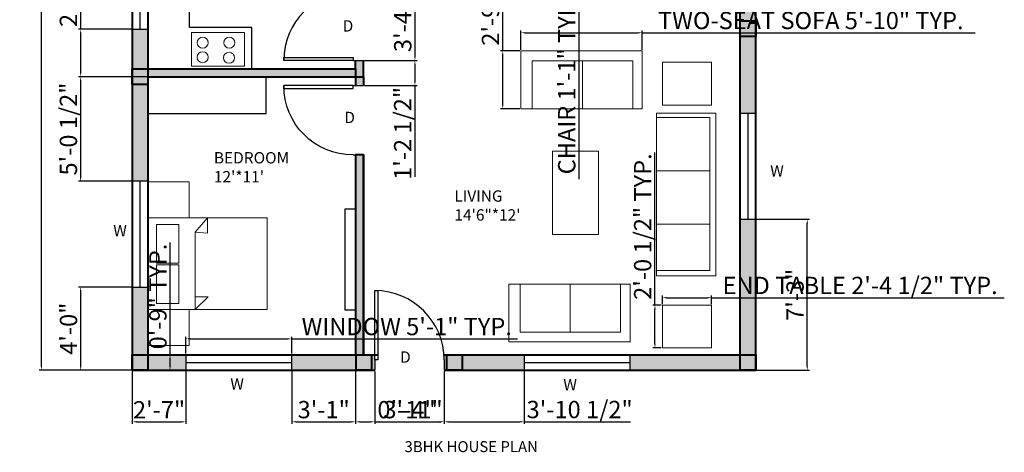
# Model space of a CAD drawing. Units: inches. Extents: x 1628 to 2197, y 2073 to 2736.
# Tile 1 of 3: x 1628 to 2197, y 2073 to 2323. Entities that reach past the tile are written whole.
import ezdxf

# ---------------------------------------------------------------- set-up
doc = ezdxf.new("R2010")
doc.units = ezdxf.units.IN
for name, color, linetype, lineweight in [('A-ANNO-DIMS', 2, 'Continuous', 18), ('A-ANNO-IDEN', 7, 'Continuous', 18), ('A-ANNO-TEXT', 7, 'Continuous', 25), ('A-AREA-IDEN', 7, 'Continuous', 18), ('A-COLS', 7, 'Continuous', 40), ('A-COLS-PATT', 8, 'Continuous', 13), ('A-EQPM', 8, 'Continuous', 18), ('A-FLOR-CASE', 8, 'Continuous', 25), ('A-FURN', 8, 'Continuous', 18), ('A-WALL-PATT', 152, 'Continuous', 13), ('bed', 210, 'Continuous', 18), ('door', 52, 'Continuous', 25), ('sofa', 190, 'Continuous', 18), ('wall', 151, 'Continuous', 40), ('window', 20, 'Continuous', 25)]:
    doc.layers.add(name, color=color, linetype=linetype, lineweight=lineweight)
doc.styles.get("Standard").update_dxf_attribs({"font": 'arial.ttf'})
doc.dimstyles.new('ISO-25', dxfattribs={"dimtxt": 10, "dimasz": 2.5, "dimexe": 1.25, "dimexo": 0.625, "dimtad": 1, "dimdec": 0, "dimlunit": 4, "dimtxsty": 'Standard', "dimcen": 2.5, "dimadec": 0, "dimazin": 0, "dimtfac": 1, "dimtdec": 0, "dimtmove": 0, "dimatfit": 3, "dimfxl": 1, "dimarcsym": 0})

# ---------------------------------------------------------------- blocks, each defined once
blk = doc.blocks.new('*U2')
for p, q in [((0, 0), (0, -6)), ((40, 0), (40, -6))]:
    blk.add_line(p, q)
blk.add_lwpolyline([(0, 0), (0, 40), (1.75, 40), (1.75, 0)], close=True)
blk.add_arc((0, 0), 40, 0, 90)
blk = doc.blocks.new('*D6')
at = {"layer": 'A-ANNO-DIMS', "color": 0, "lineweight": -2, "transparency": 16777216}
for p, q in [((1692.49, 2600.7), (1639.45, 2600.7)), ((1640.7, 2123.2), (1640.7, 2598.2)), ((1692.49, 2120.7), (1639.45, 2120.7))]:
    blk.add_line(p, q, dxfattribs=at)
at = {"layer": 'A-ANNO-DIMS', "color": 0, "transparency": 16777216}
for points in [[(1640.28, 2598.2), (1641.11, 2598.2), (1640.7, 2600.7)], [(1640.28, 2123.2), (1641.11, 2123.2), (1640.7, 2120.7)]]:
    blk.add_solid(points, dxfattribs=at)
at = {"layer": 'Defpoints', "color": 0, "transparency": 16777216}
for p in [(1640.7, 2600.7), (1693.11, 2600.7), (1693.11, 2120.7)]:
    blk.add_point(p, dxfattribs=at)
at = {"layer": 'A-ANNO-DIMS', "color": 0, "transparency": 16777216, "insert": (1634.96, 2360.7), "char_height": 10, "attachment_point": 5, "rotation": 90}
blk.add_mtext("40'", dxfattribs=at)
blk = doc.blocks.new('BED-DOUBLE-WITH-NIGHTSTANDS')
for p, q in [((27.37, 65.6), (34.42, 73.72)), ((34.42, 73.72), (34.42, 64.86)), ((27.37, 28.24), (27.37, 65.6)), ((34.42, 64.86), (27.37, 65.6)), ((27.37, 28.24), (27.37, 20.94)), ((27.37, 20.94), (34.96, 28.24)), ((34.96, 28.24), (27.37, 28.24))]:
    blk.add_line(p, q)
for points in [[(0, 73.72), (23.98, 73.72), (23.98, 94.66), (0, 94.66)], [(0, 20.94), (68.84, 20.94), (68.84, 73.72), (0, 73.72)], [(4.97, 47.66), (17.93, 47.66), (17.93, 70.03), (4.97, 70.03)], [(4.97, 24.36), (17.93, 24.36), (17.93, 46.73), (4.97, 46.73)], [(0, 0), (23.98, 0), (23.98, 20.94), (0, 20.94)]]:
    blk.add_lwpolyline(points, close=True)
blk = doc.blocks.new('SOFA-TWO-SEAT')
for p, q in [((0, 0), (0, 33.36)), ((0, 33.36), (70, 33.36)), ((70, 33.36), (70, 0)), ((35.49, 27.75), (35.49, 0)), ((6.45, 0), (0, 0)), ((70, 0), (54.71, 0))]:
    blk.add_line(p, q)
blk.add_lwpolyline([(64.53, 27.75), (6.45, 27.75), (6.45, 0), (64.53, 0)], close=True)
blk = doc.blocks.new('TABLE-END')
blk.add_lwpolyline([(28.46, 0), (0, 0), (0, 24.71), (28.46, 24.71)], close=True)
blk = doc.blocks.new('WINDOW-61IN')
blk.add_line((0, 4.5), (61.1, 4.5))
blk.add_lwpolyline([(0, 0), (61.1, 0), (61.1, 9), (0, 9)], close=True)
blk = doc.blocks.new('COLUMN-9X9')
blk.add_lwpolyline([(0, 9), (9, 9), (9, 0), (0, 0)], close=True)
blk = doc.blocks.new('*D15')
at = {"layer": 'A-ANNO-DIMS', "color": 0, "lineweight": -2, "transparency": 16777216}
for p, q in [((1724.14, 2130.33), (1724.14, 2140.12)), ((1726.64, 2138.87), (1782.75, 2138.87)), ((1785.25, 2130.33), (1785.25, 2140.12)), ((1785.25, 2138.87), (1915.54, 2138.87))]:
    blk.add_line(p, q, dxfattribs=at)
at = {"layer": 'A-ANNO-DIMS', "color": 0, "transparency": 16777216}
for points in [[(1726.64, 2139.28), (1726.64, 2138.45), (1724.14, 2138.87)], [(1782.75, 2139.28), (1782.75, 2138.45), (1785.25, 2138.87)]]:
    blk.add_solid(points, dxfattribs=at)
at = {"layer": 'Defpoints', "color": 0, "transparency": 16777216}
for p in [(1785.25, 2138.87), (1724.14, 2129.7), (1785.25, 2129.7)]:
    blk.add_point(p, dxfattribs=at)
at = {"layer": 'A-ANNO-DIMS', "color": 0, "transparency": 16777216, "insert": (1851.64, 2144.67), "char_height": 10, "attachment_point": 5}
blk.add_mtext('WINDOW 5\'-1" TYP.', dxfattribs=at)
blk = doc.blocks.new('*D16')
at = {"layer": 'A-ANNO-DIMS', "color": 0, "lineweight": -2, "transparency": 16777216}
for p, q in [((1714.98, 2129.7), (1714.98, 2194.41)), ((1723.52, 2129.7), (1713.73, 2129.7)), ((1714.98, 2123.2), (1714.98, 2127.2)), ((1723.52, 2120.7), (1713.73, 2120.7))]:
    blk.add_line(p, q, dxfattribs=at)
at = {"layer": 'A-ANNO-DIMS', "color": 0, "transparency": 16777216}
for points in [[(1714.56, 2127.2), (1715.39, 2127.2), (1714.98, 2129.7)], [(1714.56, 2123.2), (1715.39, 2123.2), (1714.98, 2120.7)]]:
    blk.add_solid(points, dxfattribs=at)
at = {"layer": 'Defpoints', "color": 0, "transparency": 16777216}
for p in [(1714.98, 2129.7), (1724.14, 2129.7), (1724.14, 2120.7)]:
    blk.add_point(p, dxfattribs=at)
at = {"layer": 'A-ANNO-DIMS', "color": 0, "transparency": 16777216, "insert": (1709.25, 2163.3), "char_height": 10, "attachment_point": 5, "rotation": 90}
blk.add_mtext('0\'-9" TYP.', dxfattribs=at)
blk = doc.blocks.new('*D17')
at = {"layer": 'A-ANNO-DIMS', "color": 0, "lineweight": -2, "transparency": 16777216}
for p, q in [((1949.73, 2356.08), (1952.33, 2356.08)), ((1951.08, 2353.58), (1951.08, 2345.41)), ((1949.73, 2342.91), (1952.33, 2342.91)), ((1951.08, 2342.91), (1951.08, 2230.98))]:
    blk.add_line(p, q, dxfattribs=at)
at = {"layer": 'A-ANNO-DIMS', "color": 0, "transparency": 16777216}
for points in [[(1950.66, 2353.58), (1951.5, 2353.58), (1951.08, 2356.08)], [(1950.66, 2345.41), (1951.5, 2345.41), (1951.08, 2342.91)]]:
    blk.add_solid(points, dxfattribs=at)
at = {"layer": 'Defpoints', "color": 0, "transparency": 16777216}
for p in [(1949.11, 2356.08), (1949.11, 2342.91), (1951.08, 2342.91)]:
    blk.add_point(p, dxfattribs=at)
at = {"layer": 'A-ANNO-DIMS', "color": 0, "transparency": 16777216, "insert": (1945.29, 2285.7), "char_height": 10, "attachment_point": 5, "rotation": 90}
blk.add_mtext('CHAIR 1\'-1" TYP.', dxfattribs=at)
blk = doc.blocks.new('*D21')
at = {"layer": 'A-ANNO-DIMS', "color": 0, "lineweight": -2, "transparency": 16777216}
for p, q in [((1999.21, 2158.97), (1999.21, 2163.86)), ((2001.71, 2162.61), (2025.17, 2162.61)), ((2027.67, 2158.97), (2027.67, 2163.86)), ((2027.67, 2162.61), (2196.66, 2162.61))]:
    blk.add_line(p, q, dxfattribs=at)
at = {"layer": 'A-ANNO-DIMS', "color": 0, "transparency": 16777216}
for points in [[(2001.71, 2163.03), (2001.71, 2162.2), (1999.21, 2162.61)], [(2025.17, 2163.03), (2025.17, 2162.2), (2027.67, 2162.61)]]:
    blk.add_solid(points, dxfattribs=at)
at = {"layer": 'Defpoints', "color": 0, "transparency": 16777216}
for p in [(2027.67, 2162.61), (1999.21, 2158.35), (2027.67, 2158.35)]:
    blk.add_point(p, dxfattribs=at)
at = {"layer": 'A-ANNO-DIMS', "color": 0, "transparency": 16777216, "insert": (2113.41, 2168.41), "char_height": 10, "attachment_point": 5}
blk.add_mtext('END TABLE 2\'-4 1/2" TYP.', dxfattribs=at)
blk = doc.blocks.new('*D22')
at = {"layer": 'A-ANNO-DIMS', "color": 0, "lineweight": -2, "transparency": 16777216}
for p, q in [((1994.94, 2158.35), (1994.94, 2246.52)), ((1998.58, 2158.35), (1993.69, 2158.35)), ((1994.94, 2136.14), (1994.94, 2155.85)), ((1998.58, 2133.64), (1993.69, 2133.64))]:
    blk.add_line(p, q, dxfattribs=at)
at = {"layer": 'A-ANNO-DIMS', "color": 0, "transparency": 16777216}
for points in [[(1994.52, 2155.85), (1995.36, 2155.85), (1994.94, 2158.35)], [(1994.52, 2136.14), (1995.36, 2136.14), (1994.94, 2133.64)]]:
    blk.add_solid(points, dxfattribs=at)
at = {"layer": 'Defpoints', "color": 0, "transparency": 16777216}
for p in [(1994.94, 2158.35), (1999.21, 2158.35), (1999.21, 2133.64)]:
    blk.add_point(p, dxfattribs=at)
at = {"layer": 'A-ANNO-DIMS', "color": 0, "transparency": 16777216, "insert": (1989.14, 2203.68), "char_height": 10, "attachment_point": 5, "rotation": 90}
blk.add_mtext('2\'-0 1/2" TYP.', dxfattribs=at)
blk = doc.blocks.new('*D23')
at = {"layer": 'A-ANNO-DIMS', "color": 0, "lineweight": -2, "transparency": 16777216}
for p, q in [((1917.57, 2305.72), (1917.57, 2316.85)), ((1920.07, 2315.6), (1985.07, 2315.6)), ((1987.57, 2305.72), (1987.57, 2316.85)), ((1987.57, 2315.6), (2179.82, 2315.6))]:
    blk.add_line(p, q, dxfattribs=at)
at = {"layer": 'A-ANNO-DIMS', "color": 0, "transparency": 16777216}
for points in [[(1920.07, 2316.01), (1920.07, 2315.18), (1917.57, 2315.6)], [(1985.07, 2316.01), (1985.07, 2315.18), (1987.57, 2315.6)]]:
    blk.add_solid(points, dxfattribs=at)
at = {"layer": 'Defpoints', "color": 0, "transparency": 16777216}
for p in [(1987.57, 2315.6), (1917.57, 2305.1), (1987.57, 2305.1)]:
    blk.add_point(p, dxfattribs=at)
at = {"layer": 'A-ANNO-DIMS', "color": 0, "transparency": 16777216, "insert": (2084.94, 2321.4), "char_height": 10, "attachment_point": 5}
blk.add_mtext('TWO-SEAT SOFA 5\'-10" TYP.', dxfattribs=at)
blk = doc.blocks.new('*D24')
at = {"layer": 'A-ANNO-DIMS', "color": 0, "lineweight": -2, "transparency": 16777216}
for p, q in [((1907.07, 2305.1), (1907.07, 2393.27)), ((1916.95, 2305.1), (1905.82, 2305.1)), ((1907.07, 2274.24), (1907.07, 2302.6)), ((1916.95, 2271.74), (1905.82, 2271.74))]:
    blk.add_line(p, q, dxfattribs=at)
at = {"layer": 'A-ANNO-DIMS', "color": 0, "transparency": 16777216}
for points in [[(1906.65, 2302.6), (1907.49, 2302.6), (1907.07, 2305.1)], [(1906.65, 2274.24), (1907.49, 2274.24), (1907.07, 2271.74)]]:
    blk.add_solid(points, dxfattribs=at)
at = {"layer": 'Defpoints', "color": 0, "transparency": 16777216}
for p in [(1907.07, 2305.1), (1917.57, 2305.1), (1917.57, 2271.74)]:
    blk.add_point(p, dxfattribs=at)
at = {"layer": 'A-ANNO-DIMS', "color": 0, "transparency": 16777216, "insert": (1901.28, 2350.44), "char_height": 10, "attachment_point": 5, "rotation": 90}
blk.add_mtext('2\'-9 1/2" TYP.', dxfattribs=at)
blk = doc.blocks.new('*D28')
at = {"layer": 'A-ANNO-DIMS', "color": 0, "lineweight": -2, "transparency": 16777216}
for p, q in [((1693.11, 2120.08), (1693.11, 2089.7)), ((1724.14, 2120.08), (1724.14, 2089.7)), ((1695.61, 2090.95), (1721.64, 2090.95))]:
    blk.add_line(p, q, dxfattribs=at)
at = {"layer": 'A-ANNO-DIMS', "color": 0, "transparency": 16777216}
for points in [[(1695.61, 2091.37), (1695.61, 2090.54), (1693.11, 2090.95)], [(1721.64, 2091.37), (1721.64, 2090.54), (1724.14, 2090.95)]]:
    blk.add_solid(points, dxfattribs=at)
at = {"layer": 'Defpoints', "color": 0, "transparency": 16777216}
for p in [(1693.11, 2120.7), (1724.14, 2120.7), (1724.14, 2090.95)]:
    blk.add_point(p, dxfattribs=at)
at = {"layer": 'A-ANNO-DIMS', "color": 0, "transparency": 16777216, "insert": (1708.63, 2096.6), "char_height": 10, "attachment_point": 5}
blk.add_mtext('2\'-7"', dxfattribs=at)
blk = doc.blocks.new('*D29')
at = {"layer": 'A-ANNO-DIMS', "color": 0, "lineweight": -2, "transparency": 16777216}
for p, q in [((1822.11, 2129.08), (1822.11, 2089.7)), ((1785.25, 2120.08), (1785.25, 2089.7)), ((1787.75, 2090.95), (1819.61, 2090.95))]:
    blk.add_line(p, q, dxfattribs=at)
at = {"layer": 'A-ANNO-DIMS', "color": 0, "transparency": 16777216}
for points in [[(1787.75, 2091.37), (1787.75, 2090.54), (1785.25, 2090.95)], [(1819.61, 2091.37), (1819.61, 2090.54), (1822.11, 2090.95)]]:
    blk.add_solid(points, dxfattribs=at)
at = {"layer": 'Defpoints', "color": 0, "transparency": 16777216}
for p in [(1822.11, 2129.7), (1785.25, 2120.7), (1822.11, 2090.95)]:
    blk.add_point(p, dxfattribs=at)
at = {"layer": 'A-ANNO-DIMS', "color": 0, "transparency": 16777216, "insert": (1803.68, 2096.69), "char_height": 10, "attachment_point": 5}
blk.add_mtext('3\'-1"', dxfattribs=at)
blk = doc.blocks.new('*D30')
at = {"layer": 'A-ANNO-DIMS', "color": 0, "lineweight": -2, "transparency": 16777216}
for p, q in [((1822.11, 2129.08), (1822.11, 2089.7)), ((1833.23, 2120.08), (1833.23, 2089.7)), ((1824.61, 2090.95), (1830.73, 2090.95)), ((1833.23, 2090.95), (1871.33, 2090.95))]:
    blk.add_line(p, q, dxfattribs=at)
at = {"layer": 'A-ANNO-DIMS', "color": 0, "transparency": 16777216}
for points in [[(1824.61, 2091.37), (1824.61, 2090.54), (1822.11, 2090.95)], [(1830.73, 2091.37), (1830.73, 2090.54), (1833.23, 2090.95)]]:
    blk.add_solid(points, dxfattribs=at)
at = {"layer": 'Defpoints', "color": 0, "transparency": 16777216}
for p in [(1822.11, 2129.7), (1833.23, 2120.7), (1833.23, 2090.95)]:
    blk.add_point(p, dxfattribs=at)
at = {"layer": 'A-ANNO-DIMS', "color": 0, "transparency": 16777216, "insert": (1853.53, 2096.68), "char_height": 10, "attachment_point": 5}
blk.add_mtext('0\'-11"', dxfattribs=at)
blk = doc.blocks.new('*D31')
at = {"layer": 'A-ANNO-DIMS', "color": 0, "lineweight": -2, "transparency": 16777216}
for p, q in [((1833.23, 2120.08), (1833.23, 2089.7)), ((1873.23, 2120.08), (1873.23, 2089.7)), ((1835.73, 2090.95), (1870.73, 2090.95))]:
    blk.add_line(p, q, dxfattribs=at)
at = {"layer": 'A-ANNO-DIMS', "color": 0, "transparency": 16777216}
for points in [[(1835.73, 2091.37), (1835.73, 2090.54), (1833.23, 2090.95)], [(1870.73, 2091.37), (1870.73, 2090.54), (1873.23, 2090.95)]]:
    blk.add_solid(points, dxfattribs=at)
at = {"layer": 'Defpoints', "color": 0, "transparency": 16777216}
for p in [(1833.23, 2120.7), (1873.23, 2120.7), (1873.23, 2090.95)]:
    blk.add_point(p, dxfattribs=at)
at = {"layer": 'A-ANNO-DIMS', "color": 0, "transparency": 16777216, "insert": (1853.23, 2096.69), "char_height": 10, "attachment_point": 5}
blk.add_mtext('3\'-4"', dxfattribs=at)
blk = doc.blocks.new('*D32')
at = {"layer": 'A-ANNO-DIMS', "color": 0, "lineweight": -2, "transparency": 16777216}
for p, q in [((1873.23, 2120.08), (1873.23, 2089.7)), ((1919.51, 2120.08), (1919.51, 2089.7)), ((1875.73, 2090.95), (1917.01, 2090.95)), ((1919.51, 2090.95), (1980.91, 2090.95))]:
    blk.add_line(p, q, dxfattribs=at)
at = {"layer": 'A-ANNO-DIMS', "color": 0, "transparency": 16777216}
for points in [[(1875.73, 2091.37), (1875.73, 2090.54), (1873.23, 2090.95)], [(1917.01, 2091.37), (1917.01, 2090.54), (1919.51, 2090.95)]]:
    blk.add_solid(points, dxfattribs=at)
at = {"layer": 'Defpoints', "color": 0, "transparency": 16777216}
for p in [(1873.23, 2120.7), (1919.51, 2120.7), (1919.51, 2090.95)]:
    blk.add_point(p, dxfattribs=at)
at = {"layer": 'A-ANNO-DIMS', "color": 0, "transparency": 16777216, "insert": (1951.46, 2096.75), "char_height": 10, "attachment_point": 5}
blk.add_mtext('3\'-10 1/2"', dxfattribs=at)
blk = doc.blocks.new('*D33')
at = {"layer": 'A-ANNO-DIMS', "color": 0, "lineweight": -2, "transparency": 16777216}
for p, q in [((1692.49, 2168.74), (1662.11, 2168.74)), ((1663.36, 2123.2), (1663.36, 2166.24)), ((1692.49, 2120.7), (1662.11, 2120.7))]:
    blk.add_line(p, q, dxfattribs=at)
at = {"layer": 'A-ANNO-DIMS', "color": 0, "transparency": 16777216}
for points in [[(1662.94, 2166.24), (1663.78, 2166.24), (1663.36, 2168.74)], [(1662.94, 2123.2), (1663.78, 2123.2), (1663.36, 2120.7)]]:
    blk.add_solid(points, dxfattribs=at)
at = {"layer": 'Defpoints', "color": 0, "transparency": 16777216}
for p in [(1663.36, 2168.74), (1693.11, 2168.74), (1693.11, 2120.7)]:
    blk.add_point(p, dxfattribs=at)
at = {"layer": 'A-ANNO-DIMS', "color": 0, "transparency": 16777216, "insert": (1657.63, 2144.72), "char_height": 10, "attachment_point": 5, "rotation": 90}
blk.add_mtext('4\'-0"', dxfattribs=at)
blk = doc.blocks.new('*D34')
at = {"layer": 'A-ANNO-DIMS', "color": 0, "lineweight": -2, "transparency": 16777216}
for p, q in [((1701.49, 2290.2), (1662.11, 2290.2)), ((1663.36, 2232.34), (1663.36, 2287.7)), ((1692.49, 2229.84), (1662.11, 2229.84))]:
    blk.add_line(p, q, dxfattribs=at)
at = {"layer": 'A-ANNO-DIMS', "color": 0, "transparency": 16777216}
for points in [[(1662.94, 2287.7), (1663.78, 2287.7), (1663.36, 2290.2)], [(1662.94, 2232.34), (1663.78, 2232.34), (1663.36, 2229.84)]]:
    blk.add_solid(points, dxfattribs=at)
at = {"layer": 'Defpoints', "color": 0, "transparency": 16777216}
for p in [(1663.36, 2290.2), (1702.11, 2290.2), (1693.11, 2229.84)]:
    blk.add_point(p, dxfattribs=at)
at = {"layer": 'A-ANNO-DIMS', "color": 0, "transparency": 16777216, "insert": (1657.57, 2260.02), "char_height": 10, "attachment_point": 5, "rotation": 90}
blk.add_mtext('5\'-0 1/2"', dxfattribs=at)
blk = doc.blocks.new('*D35')
at = {"layer": 'A-ANNO-DIMS', "color": 0, "lineweight": -2, "transparency": 16777216}
for p, q in [((1663.36, 2317.65), (1663.36, 2371.45)), ((1692.49, 2317.65), (1662.11, 2317.65)), ((1663.36, 2292.7), (1663.36, 2315.15)), ((1701.49, 2290.2), (1662.11, 2290.2))]:
    blk.add_line(p, q, dxfattribs=at)
at = {"layer": 'A-ANNO-DIMS', "color": 0, "transparency": 16777216}
for points in [[(1662.94, 2315.15), (1663.78, 2315.15), (1663.36, 2317.65)], [(1662.94, 2292.7), (1663.78, 2292.7), (1663.36, 2290.2)]]:
    blk.add_solid(points, dxfattribs=at)
at = {"layer": 'Defpoints', "color": 0, "transparency": 16777216}
for p in [(1663.36, 2317.65), (1693.11, 2317.65), (1702.11, 2290.2)]:
    blk.add_point(p, dxfattribs=at)
at = {"layer": 'A-ANNO-DIMS', "color": 0, "transparency": 16777216, "insert": (1657.56, 2345.8), "char_height": 10, "attachment_point": 5, "rotation": 90}
blk.add_mtext('2\'-3 1/2"', dxfattribs=at)
blk = doc.blocks.new('*D41')
at = {"layer": 'A-ANNO-DIMS', "color": 0, "lineweight": -2, "transparency": 16777216}
for p, q in [((2053.74, 2207.91), (2084.11, 2207.91)), ((2082.86, 2123.2), (2082.86, 2205.41)), ((2053.74, 2120.7), (2084.11, 2120.7))]:
    blk.add_line(p, q, dxfattribs=at)
at = {"layer": 'A-ANNO-DIMS', "color": 0, "transparency": 16777216}
for points in [[(2082.44, 2205.41), (2083.28, 2205.41), (2082.86, 2207.91)], [(2082.44, 2123.2), (2083.28, 2123.2), (2082.86, 2120.7)]]:
    blk.add_solid(points, dxfattribs=at)
at = {"layer": 'Defpoints', "color": 0, "transparency": 16777216}
for p in [(2053.11, 2207.91), (2082.86, 2207.91), (2053.11, 2120.7)]:
    blk.add_point(p, dxfattribs=at)
at = {"layer": 'A-ANNO-DIMS', "color": 0, "transparency": 16777216, "insert": (2077.13, 2164.31), "char_height": 10, "attachment_point": 5, "rotation": 90}
blk.add_mtext('7\'-3"', dxfattribs=at)
blk = doc.blocks.new('*D52')
at = {"layer": 'A-ANNO-DIMS', "color": 0, "lineweight": -2, "transparency": 16777216}
for p, q in [((1827.24, 2299.52), (1857.61, 2299.52)), ((1856.36, 2297.02), (1856.36, 2287.58)), ((1827.24, 2285.08), (1857.61, 2285.08)), ((1856.36, 2285.08), (1856.36, 2232.39))]:
    blk.add_line(p, q, dxfattribs=at)
at = {"layer": 'A-ANNO-DIMS', "color": 0, "transparency": 16777216}
for points in [[(1855.94, 2297.02), (1856.78, 2297.02), (1856.36, 2299.52)], [(1855.94, 2287.58), (1856.78, 2287.58), (1856.36, 2285.08)]]:
    blk.add_solid(points, dxfattribs=at)
at = {"layer": 'Defpoints', "color": 0, "transparency": 16777216}
for p in [(1826.61, 2299.52), (1826.61, 2285.08), (1856.36, 2285.08)]:
    blk.add_point(p, dxfattribs=at)
at = {"layer": 'A-ANNO-DIMS', "color": 0, "transparency": 16777216, "insert": (1850.57, 2257.49), "char_height": 10, "attachment_point": 5, "rotation": 90}
blk.add_mtext('1\'-2 1/2"', dxfattribs=at)
blk = doc.blocks.new('*D53')
at = {"layer": 'A-ANNO-DIMS', "color": 0, "lineweight": -2, "transparency": 16777216}
for p, q in [((1827.24, 2339.52), (1857.61, 2339.52)), ((1856.36, 2337.02), (1856.36, 2302.02)), ((1827.24, 2299.52), (1857.61, 2299.52))]:
    blk.add_line(p, q, dxfattribs=at)
at = {"layer": 'A-ANNO-DIMS', "color": 0, "transparency": 16777216}
for points in [[(1855.94, 2337.02), (1856.78, 2337.02), (1856.36, 2339.52)], [(1855.94, 2302.02), (1856.78, 2302.02), (1856.36, 2299.52)]]:
    blk.add_solid(points, dxfattribs=at)
at = {"layer": 'Defpoints', "color": 0, "transparency": 16777216}
for p in [(1826.61, 2339.52), (1826.61, 2299.52), (1856.36, 2299.52)]:
    blk.add_point(p, dxfattribs=at)
at = {"layer": 'A-ANNO-DIMS', "color": 0, "transparency": 16777216, "insert": (1850.63, 2319.52), "char_height": 10, "attachment_point": 5, "rotation": 90}
blk.add_mtext('3\'-4"', dxfattribs=at)

msp = doc.modelspace()

# ---------------------------------------------------------------- hatches: boundary and pattern name
at = {"layer": 'A-COLS-PATT'}
h = msp.add_hatch(color=256, dxfattribs=at)
h.dxf.hatch_style = 1
h.paths.add_polyline_path([(1702.11, 2600.7), (1693.11, 2600.7), (1693.11, 2591.7), (1702.11, 2591.7)])
h.paths.add_polyline_path([(1879.79, 2600.7), (1870.79, 2600.7), (1870.79, 2591.7), (1879.79, 2591.7)])
h.paths.add_polyline_path([(2053.11, 2600.7), (2044.11, 2600.7), (2044.11, 2591.7), (2053.11, 2591.7)])
h.paths.add_polyline_path([(1702.11, 2395.2), (1693.11, 2395.2), (1693.11, 2386.2), (1702.11, 2386.2)])
h.paths.add_polyline_path([(1826.61, 2395.2), (1817.61, 2395.2), (1817.61, 2386.2), (1826.61, 2386.2)])
h.paths.add_polyline_path([(1702.11, 2459.7), (1693.11, 2459.7), (1693.11, 2450.7), (1702.11, 2450.7)])
h.paths.add_polyline_path([(2053.11, 2459.7), (2044.11, 2459.7), (2044.11, 2455.2), (2053.11, 2455.2)])
h.paths.add_polyline_path([(2053.11, 2455.2), (2044.11, 2455.2), (2044.11, 2451.94), (2053.11, 2451.94)])
h.paths.add_polyline_path([(2053.11, 2460.94), (2044.11, 2460.94), (2044.11, 2459.7), (2053.11, 2459.7)])
h.paths.add_polyline_path([(2053.11, 2390.99), (2044.11, 2390.99), (2044.11, 2381.99), (2053.11, 2381.99)])
h.paths.add_polyline_path([(2053.11, 2322.52), (2044.11, 2322.52), (2044.11, 2313.52), (2053.11, 2313.52)])
h.paths.add_polyline_path([(1702.11, 2294.7), (1693.11, 2294.7), (1693.11, 2285.7), (1702.11, 2285.7)])
h.paths.add_polyline_path([(1702.11, 2129.7), (1693.11, 2129.7), (1693.11, 2120.7), (1702.11, 2120.7)])
h.paths.add_polyline_path([(1831.35, 2129.7), (1822.35, 2129.7), (1822.35, 2120.7), (1831.35, 2120.7)])
h.paths.add_polyline_path([(1883.72, 2129.7), (1874.72, 2129.7), (1874.72, 2120.7), (1883.72, 2120.7)])
h.paths.add_polyline_path([(2053.11, 2129.7), (2044.11, 2129.7), (2044.11, 2120.7), (2053.11, 2120.7)])
at = {"layer": 'A-WALL-PATT'}
h = msp.add_hatch(color=256, dxfattribs=at)
h.dxf.hatch_style = 1
h.paths.add_polyline_path([(1753.01, 2600.7), (1702.11, 2600.7), (1702.11, 2591.7), (1753.01, 2591.7)])
h.paths.add_polyline_path([(1870.79, 2600.7), (1814.12, 2600.7), (1814.12, 2591.7), (1870.79, 2591.7)])
h.paths.add_polyline_path([(1948.37, 2600.7), (1879.79, 2600.7), (1879.79, 2591.7), (1909.32, 2591.7), (1948.37, 2591.7)])
h.paths.add_polyline_path([(2044.11, 2600.7), (2009.47, 2600.7), (2009.47, 2591.7), (2044.11, 2591.7)])
h.paths.add_polyline_path([(2053.11, 2591.7), (2044.11, 2591.7), (2044.11, 2550.07), (2053.11, 2550.07)])
h.paths.add_polyline_path([(1702.11, 2591.7), (1693.11, 2591.7), (1693.11, 2549.95), (1702.11, 2549.95)])
h.paths.add_polyline_path([(1702.11, 2488.85), (1693.11, 2488.85), (1693.11, 2459.7), (1702.11, 2459.7)])
h.paths.add_polyline_path([(1828.05, 2459.7), (1702.11, 2459.7), (1702.11, 2455.2), (1733.61, 2455.2), (1792.11, 2455.2), (1828.05, 2455.2)])
h.paths.add_polyline_path([(1885.43, 2459.7), (1868.05, 2459.7), (1868.05, 2455.2), (1885.43, 2455.2)])
h.paths.add_polyline_path([(2053.11, 2488.97), (2044.11, 2488.97), (2044.11, 2474.68), (2044.11, 2460.94), (2053.11, 2460.94)])
h.paths.add_polyline_path([(2053.11, 2451.94), (2044.11, 2451.94), (2044.11, 2437.29), (2053.11, 2437.29)])
h.paths.add_polyline_path([(2053.11, 2414.88), (2044.11, 2414.88), (2044.11, 2390.99), (2053.11, 2390.99)])
h.paths.add_polyline_path([(2044.11, 2459.7), (1925.43, 2459.7), (1925.43, 2455.2), (2044.11, 2455.2)])
h.paths.add_polyline_path([(2053.11, 2381.99), (2044.11, 2381.99), (2044.11, 2322.52), (2053.11, 2322.52)])
h.paths.add_polyline_path([(1919.51, 2129.7), (1883.72, 2129.7), (1883.72, 2120.7), (1919.51, 2120.7)])
h.paths.add_polyline_path([(2044.11, 2129.7), (1980.61, 2129.7), (1980.61, 2120.7), (2044.11, 2120.7)])
h.paths.add_polyline_path([(2053.11, 2207.91), (2044.11, 2207.91), (2044.11, 2129.7), (2053.11, 2129.7)])
h.paths.add_polyline_path([(2053.11, 2313.52), (2044.11, 2313.52), (2044.11, 2269.02), (2053.11, 2269.02)])
h.paths.add_polyline_path([(1822.35, 2129.7), (1785.25, 2129.7), (1785.25, 2120.7), (1822.35, 2120.7)])
h.paths.add_polyline_path([(1724.14, 2129.7), (1702.11, 2129.7), (1702.11, 2120.7), (1724.14, 2120.7)])
h.paths.add_polyline_path([(1702.11, 2168.74), (1693.11, 2168.74), (1693.11, 2129.7), (1702.11, 2129.7)])
h.paths.add_polyline_path([(1702.11, 2285.7), (1693.11, 2285.7), (1693.11, 2229.84), (1702.11, 2229.84)])
h.paths.add_polyline_path([(1702.11, 2317.65), (1693.11, 2317.65), (1693.11, 2294.7), (1702.11, 2294.7)])
h.paths.add_polyline_path([(1702.11, 2386.2), (1693.11, 2386.2), (1693.11, 2378.75), (1702.11, 2378.75)])
h.paths.add_polyline_path([(2044.11, 2389.2), (1938.65, 2389.2), (1938.65, 2384.7), (2044.11, 2384.7)])
h.paths.add_polyline_path([(1817.61, 2395.2), (1782.07, 2395.2), (1702.11, 2395.2), (1702.11, 2390.7), (1796.61, 2390.7), (1817.61, 2390.7)])
h.paths.add_polyline_path([(1796.61, 2397.27), (1792.11, 2397.27), (1792.11, 2395.2), (1796.61, 2395.2)])
h.paths.add_polyline_path([(1826.61, 2386.2), (1822.11, 2386.2), (1822.11, 2339.52), (1826.61, 2339.52)])
h.paths.add_polyline_path([(1826.61, 2299.52), (1822.11, 2299.52), (1822.11, 2294.7), (1822.11, 2290.2), (1826.61, 2290.2)])
h.paths.add_polyline_path([(1826.61, 2290.2), (1822.11, 2290.2), (1822.11, 2285.08), (1826.61, 2285.08)])
h.paths.add_polyline_path([(1822.11, 2294.7), (1702.11, 2294.7), (1702.11, 2290.2), (1770.51, 2290.2), (1822.11, 2290.2)])
h.paths.add_polyline_path([(1693.11, 2437.86), (1702.11, 2437.86), (1702.11, 2450.7), (1693.11, 2450.7)])
h.paths.add_polyline_path([(1702.11, 2410.6), (1693.11, 2410.6), (1693.11, 2395.2), (1702.11, 2395.2)])
h = msp.add_hatch(color=256, dxfattribs=at)
h.dxf.hatch_style = 1
h.paths.add_polyline_path([(1826.61, 2245.08), (1822.11, 2245.08), (1822.11, 2129.7), (1826.61, 2129.7)])
h.paths.add_polyline_path([(1833.23, 2126.7), (1833.23, 2129.7), (1831.35, 2129.7), (1831.35, 2120.7), (1833.23, 2120.7)])
h.paths.add_polyline_path([(1874.72, 2129.7), (1873.11, 2129.7, -0.01877), (1873.23, 2126.7), (1873.23, 2120.7), (1874.72, 2120.7)])

# ---------------------------------------------------------------- linework, layer by layer
at = {"layer": 'A-EQPM'}
msp.add_lwpolyline([(1757.99, 2296.27), (1727.31, 2296.27), (1727.31, 2315.73), (1757.99, 2315.73)], close=True, dxfattribs=at)
for centre in [(1733.79, 2309.87), (1749.19, 2309.87), (1733.79, 2301.5), (1749.05, 2301.15)]:
    msp.add_circle(centre, 3.19, dxfattribs=at)
at = {"layer": 'A-FLOR-CASE'}
for p, q in [((1726.11, 2318.7), (1726.11, 2366.7)), ((1762.11, 2318.7), (1726.11, 2318.7)), ((1762.11, 2294.7), (1762.11, 2318.7)), ((1702.11, 2294.7), (1726.11, 2294.7))]:
    msp.add_line(p, q, dxfattribs=at)
for points in [[(1770.51, 2290.2), (1702.11, 2290.2), (1702.11, 2269.04), (1770.51, 2269.04)], [(1822.11, 2213.69), (1815.98, 2213.69), (1815.98, 2155.71), (1822.11, 2155.71)]]:
    msp.add_lwpolyline(points, close=True, dxfattribs=at)
at = {"layer": 'A-FURN'}
msp.add_lwpolyline([(1935.83, 2199.15), (1962.37, 2199.15), (1962.37, 2247.3), (1935.83, 2247.3)], close=True, dxfattribs=at)
at = {"layer": 'sofa'}
for p, q in [((2030.17, 2269.22), (1995.89, 2269.22)), ((1995.89, 2269.22), (1995.89, 2265.48)), ((2030.17, 2175.28), (2030.17, 2269.22)), ((2026.69, 2235.81), (1995.89, 2235.81)), ((2026.69, 2205.07), (1995.89, 2205.07)), ((1995.89, 2178.42), (1995.89, 2175.28)), ((1995.89, 2175.28), (2030.17, 2175.28))]:
    msp.add_line(p, q, dxfattribs=at)
msp.add_lwpolyline([(2026.69, 2178.42), (1995.89, 2178.42), (1995.89, 2266.77), (2026.69, 2266.77)], close=True, dxfattribs=at)
at = {"layer": 'wall'}
for p, q in [((1702.11, 2390.7), (1702.11, 2294.7)), ((1822.11, 2294.7), (1822.11, 2299.52)), ((1826.61, 2290.2), (1826.61, 2299.52)), ((1702.11, 2294.7), (1822.11, 2294.7)), ((1822.11, 2294.7), (1822.11, 2285.08)), ((1702.11, 2290.2), (1826.61, 2290.2)), ((1826.61, 2290.2), (1826.61, 2285.08)), ((1822.11, 2245.08), (1822.11, 2129.7)), ((1826.61, 2245.08), (1826.61, 2129.7))]:
    msp.add_line(p, q, dxfattribs=at)
for points in [[(1873.23, 2120.7), (2053.11, 2120.7), (2053.11, 2600.7), (1693.11, 2600.7), (1693.11, 2120.7), (1833.23, 2120.7)], [(1873.11, 2129.7), (2044.11, 2129.7), (2044.11, 2591.7), (1702.11, 2591.7), (1702.11, 2129.7), (1834.98, 2129.7)]]:
    msp.add_lwpolyline(points, dxfattribs=at)
msp.add_lwpolyline([(1822.11, 2129.7), (1826.61, 2129.7), (1826.61, 2245.08), (1822.11, 2245.08)], close=True, dxfattribs=at)

# ---------------------------------------------------------------- block references
at = {"layer": 'A-COLS'}
for p in [(2044.11, 2313.52), (1693.11, 2285.7), (1693.11, 2120.7), (1822.35, 2120.7), (1874.72, 2120.7), (2044.11, 2120.7)]:
    msp.add_blockref('COLUMN-9X9', p, dxfattribs=at)
at = {"layer": 'A-FURN'}
for p in [(1999.21, 2273.83), (1999.21, 2133.64)]:
    msp.add_blockref('TABLE-END', p, dxfattribs=at)
at = {"layer": 'bed'}
msp.add_blockref('BED-DOUBLE-WITH-NIGHTSTANDS', (1702.11, 2134.95), dxfattribs=at)
at = {"layer": 'door', "rotation": 90}
msp.add_blockref('*U2', (1820.61, 2299.52), dxfattribs=at)
at = {"layer": 'door', "xscale": -1, "rotation": 90}
msp.add_blockref('*U2', (1820.61, 2285.08), dxfattribs=at)
at = {"layer": 'door'}
msp.add_blockref('*U2', (1833.23, 2126.7), dxfattribs=at)
at = {"layer": 'sofa'}
msp.add_blockref('SOFA-TWO-SEAT', (1917.57, 2271.74), dxfattribs=at)
at = {"layer": 'sofa', "extrusion": (0, 0, -1), "zscale": -1, "rotation": 180}
msp.add_blockref('SOFA-TWO-SEAT', (-1910.58, 2170.51), dxfattribs=at)
at = {"layer": 'window'}
for p, rotation in [((1693.11, 2378.75), 270.0000000000007), ((2044.11, 2269.02), 270.0000000000007), ((1693.11, 2229.84), 270.0000000000004)]:
    msp.add_blockref('WINDOW-61IN', p, dxfattribs=dict(at, rotation=rotation))
for p in [(1724.14, 2120.7), (1919.51, 2120.7)]:
    msp.add_blockref('WINDOW-61IN', p, dxfattribs=at)

# ---------------------------------------------------------------- texts
at = {"layer": 'A-ANNO-IDEN', "char_height": 6.55, "attachment_point": 1}
for s, insert in [('D', (1814.63, 2322.84)), ('D', (1815.6, 2269.96)), ('W', (2061.5, 2239.15)), ('W', (1682.17, 2204.6)), ('D', (1847.8, 2131.64)), ('W', (1749.76, 2116.13)), ('W', (1942.05, 2115.61))]:
    msp.add_mtext_dynamic_manual_height_columns(s, width=86.8171, gutter_width=32.74, heights=[0], dxfattribs=dict(at, insert=insert))
at = {"layer": 'A-ANNO-TEXT', "insert": (1850.34, 2079.79), "char_height": 6.3324, "attachment_point": 1}
msp.add_mtext_dynamic_manual_height_columns('3BHK HOUSE PLAN', width=835.9168, gutter_width=31.66, heights=[0], dxfattribs=at)
at = {"layer": 'A-AREA-IDEN', "char_height": 6.549, "attachment_point": 1}
for s, insert in [("BEDROOM\\P12'*11'", (1740.27, 2246.69)), ('LIVING\\P14\'6"*12\'', (1879.15, 2224.61))]:
    msp.add_mtext_dynamic_manual_height_columns(s, width=86.8171, gutter_width=32.74, heights=[0], dxfattribs=dict(at, insert=insert))

# ---------------------------------------------------------------- dimensions: what is measured, and where the dimension line sits
at = {"layer": 'A-ANNO-DIMS'}
for base, p1, p2, angle, override, picture, middle in [((1640.7, 2600.7), (1693.11, 2120.7), (1693.11, 2600.7), 90, {"dimclrd": 0, "dimclre": 0, "dimclrt": 0}, '*D6', (1634.96, 2360.7)), ((1663.3609, 2317.6491), (1702.1109, 2290.2024), (1693.1109, 2317.6491), 90, {"dimdec": 1, "dimlfac": 1, "dimrnd": 0, "dimzin": 1, "dimdsep": 46, "dimlunit": 4, "dimfrac": 2}, '*D35', (1657.562, 2345.8014)), ((1856.36, 2299.52), (1826.61, 2339.52), (1826.61, 2299.52), 270, {"dimdec": 1, "dimlfac": 1, "dimrnd": 0, "dimzin": 1, "dimdsep": 46, "dimlunit": 4, "dimfrac": 2}, '*D53', (1850.63, 2319.52)), ((1856.36, 2285.08), (1826.61, 2299.52), (1826.61, 2285.08), 270, {"dimdec": 1, "dimlfac": 1, "dimrnd": 0, "dimzin": 1, "dimdsep": 46, "dimlunit": 4, "dimfrac": 2}, '*D52', (1850.57, 2257.49)), ((1663.36, 2290.2), (1693.11, 2229.84), (1702.11, 2290.2), 90, {"dimdec": 1, "dimlfac": 1, "dimrnd": 0, "dimzin": 1, "dimdsep": 46, "dimlunit": 4, "dimfrac": 2}, '*D34', (1657.57, 2260.02)), ((2082.86, 2207.91), (2053.11, 2120.7), (2053.11, 2207.91), 90, {"dimdec": 1, "dimlfac": 1, "dimrnd": 0, "dimzin": 1, "dimdsep": 46, "dimlunit": 4, "dimfrac": 2}, '*D41', (2077.13, 2164.31)), ((1663.36, 2168.74), (1693.11, 2120.7), (1693.11, 2168.74), 90, {"dimdec": 1, "dimlfac": 1, "dimrnd": 0, "dimzin": 1, "dimdsep": 46, "dimlunit": 4, "dimfrac": 2}, '*D33', (1657.63, 2144.72))]:
    dim = msp.add_linear_dim(base=base, p1=p1, p2=p2, angle=angle, dimstyle='ISO-25', override=override, dxfattribs=at)
    dim.commit()
    dim.dimension.update_dxf_attribs({"geometry": picture, "text_midpoint": middle})
for base, p1, p2, angle, text, picture, middle in [((1907.07, 2305.1), (1917.57, 2271.74), (1917.57, 2305.1), 90, '<> TYP.', '*D24', (1901.28, 2350.44)), ((1951.08, 2342.91), (1949.11, 2356.08), (1949.11, 2342.91), 270, 'CHAIR <> TYP.', '*D17', (1945.29, 2285.7)), ((1994.94, 2158.35), (1999.21, 2133.64), (1999.21, 2158.35), 90, '<> TYP.', '*D22', (1989.14, 2203.68)), ((1714.98, 2129.7), (1724.14, 2120.7), (1724.14, 2129.7), 90, '<> TYP.', '*D16', (1709.25, 2163.3))]:
    dim = msp.add_linear_dim(base=base, p1=p1, p2=p2, angle=angle, text=text, dimstyle='ISO-25', override={"dimdec": 1, "dimlfac": 1, "dimrnd": 0, "dimzin": 1, "dimdsep": 46, "dimlunit": 4, "dimfrac": 2}, dxfattribs=at)
    dim.commit()
    dim.dimension.update_dxf_attribs({"geometry": picture, "text_midpoint": middle})
for base, p1, p2, text, picture, middle in [((1987.57, 2315.6), (1917.57, 2305.1), (1987.57, 2305.1), 'TWO-SEAT SOFA <> TYP.', '*D23', (2084.94, 2321.4)), ((2027.67, 2162.61), (1999.21, 2158.35), (2027.67, 2158.35), 'END TABLE <> TYP.', '*D21', (2113.41, 2168.41)), ((1785.25, 2138.87), (1724.14, 2129.7), (1785.25, 2129.7), 'WINDOW <> TYP.', '*D15', (1851.64, 2144.67))]:
    dim = msp.add_linear_dim(base=base, p1=p1, p2=p2, text=text, dimstyle='ISO-25', override={"dimdec": 1, "dimlfac": 1, "dimrnd": 0, "dimzin": 1, "dimdsep": 46, "dimlunit": 4, "dimfrac": 2}, dxfattribs=at)
    dim.commit()
    dim.dimension.update_dxf_attribs({"geometry": picture, "text_midpoint": middle})
for base, p1, p2, picture, middle in [((1822.11, 2090.95), (1785.25, 2120.7), (1822.11, 2129.7), '*D29', (1803.68, 2096.69)), ((1833.23, 2090.95), (1822.11, 2129.7), (1833.23, 2120.7), '*D30', (1853.53, 2096.68)), ((1724.14, 2090.95), (1693.11, 2120.7), (1724.14, 2120.7), '*D28', (1708.63, 2096.6)), ((1873.23, 2090.95), (1833.23, 2120.7), (1873.23, 2120.7), '*D31', (1853.23, 2096.69)), ((1919.51, 2090.95), (1873.23, 2120.7), (1919.51, 2120.7), '*D32', (1951.46, 2096.75))]:
    dim = msp.add_linear_dim(base=base, p1=p1, p2=p2, dimstyle='ISO-25', override={"dimdec": 1, "dimlfac": 1, "dimrnd": 0, "dimzin": 1, "dimdsep": 46, "dimlunit": 4, "dimfrac": 2}, dxfattribs=at)
    dim.commit()
    dim.dimension.update_dxf_attribs({"geometry": picture, "text_midpoint": middle})

doc.saveas('drawing.dxf')
